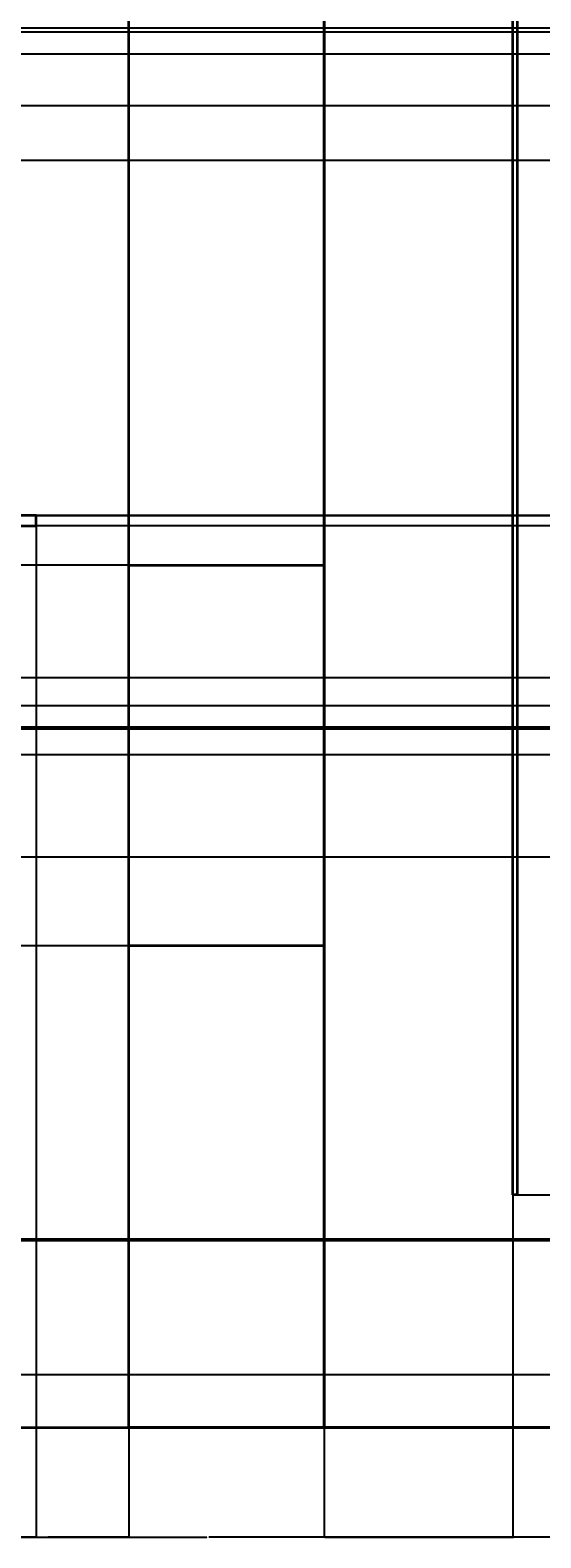
# Model space of a CAD drawing. Units: feet. Extents: x 4092 to 5585, y 725 to 1390.
# Tile 5 of 7: x 5204 to 5346, y 725 to 1146. Entities that reach past the tile are written whole.
import ezdxf

# ---------------------------------------------------------------- set-up
doc = ezdxf.new("R2010")
doc.units = ezdxf.units.FT
doc.layers.add('A-ANNO-DIMS', color=2, linetype='Continuous', lineweight=18)
doc.layers.add('A-ELEV', color=7, linetype='Continuous', lineweight=35)
doc.styles.get("Standard").update_dxf_attribs({"font": 'arial.ttf'})
doc.dimstyles.get("Standard").update_dxf_attribs({"dimtxt": 0.18, "dimasz": 0.18, "dimexe": 0.18, "dimexo": 0.0625, "dimgap": 0.09, "dimtad": 0, "dimtih": 1, "dimtoh": 1, "dimdec": 1, "dimzin": 0, "dimdsep": 46, "dimlunit": 3, "dimtxsty": 'Standard', "dimcen": 0.09, "dimadec": 0, "dimazin": 0, "dimtfac": 1, "dimtdec": 1, "dimtofl": 0, "dimtmove": 0, "dimatfit": 3, "dimfxl": 1, "dimtolj": 1, "dimtzin": 0, "dimarcsym": 0})

# ---------------------------------------------------------------- blocks, each defined once
blk = doc.blocks.new('*D4')
at = {"layer": 'A-ANNO-DIMS', "color": 0, "lineweight": -2, "transparency": 16777216}
for p, q in [((4953.29, 755.89), (4953.29, 725.07)), ((5553.29, 755.89), (5553.29, 725.07)), ((4953.47, 725.25), (5253, 725.25)), ((5553.11, 725.25), (5253.58, 725.25))]:
    blk.add_line(p, q, dxfattribs=at)
at = {"layer": 'A-ANNO-DIMS', "color": 0, "transparency": 16777216}
for points in [[(4953.47, 725.28), (4953.47, 725.22), (4953.29, 725.25)], [(5553.11, 725.28), (5553.11, 725.22), (5553.29, 725.25)]]:
    blk.add_solid(points, dxfattribs=at)
at = {"layer": 'Defpoints', "color": 0, "transparency": 16777216}
for p in [(4953.29, 755.95), (5553.29, 755.95), (5553.29, 725.25)]:
    blk.add_point(p, dxfattribs=at)
at = {"layer": 'A-ANNO-DIMS', "color": 0, "transparency": 16777216, "insert": (5253.29, 725.25), "char_height": 0.18, "attachment_point": 5}
blk.add_mtext('\\A1;600', dxfattribs=at)
blk = doc.blocks.new('*D5')
at = {"layer": 'A-ANNO-DIMS', "color": 0, "lineweight": -2, "transparency": 16777216}
for p, q in [((5264.26, 1358.97), (5584.71, 1358.97)), ((5584.53, 1358.79), (5584.53, 1057.64)), ((5584.53, 756.13), (5584.53, 1057.28)), ((5553.36, 755.95), (5584.71, 755.95))]:
    blk.add_line(p, q, dxfattribs=at)
at = {"layer": 'A-ANNO-DIMS', "color": 0, "transparency": 16777216}
for points in [[(5584.5, 1358.79), (5584.56, 1358.79), (5584.53, 1358.97)], [(5584.5, 756.13), (5584.56, 756.13), (5584.53, 755.95)]]:
    blk.add_solid(points, dxfattribs=at)
at = {"layer": 'Defpoints', "color": 0, "transparency": 16777216}
for p in [(5264.2, 1358.97), (5584.53, 1358.97), (5553.29, 755.95)]:
    blk.add_point(p, dxfattribs=at)
at = {"layer": 'A-ANNO-DIMS', "color": 0, "transparency": 16777216, "insert": (5584.53, 1057.46), "char_height": 0.18, "attachment_point": 5}
blk.add_mtext('\\A1;603', dxfattribs=at)
blk = doc.blocks.new('*D17')
at = {"layer": 'A-ANNO-DIMS', "color": 0, "lineweight": -2, "transparency": 16777216}
for p, q in [((5021.54, 951.2), (4921.27, 951.2)), ((4921.45, 951.02), (4921.45, 853.76)), ((4921.45, 756.13), (4921.45, 853.39)), ((5285.73, 755.95), (4921.27, 755.95))]:
    blk.add_line(p, q, dxfattribs=at)
at = {"layer": 'A-ANNO-DIMS', "color": 0, "transparency": 16777216}
for points in [[(4921.42, 951.02), (4921.48, 951.02), (4921.45, 951.2)], [(4921.42, 756.13), (4921.48, 756.13), (4921.45, 755.95)]]:
    blk.add_solid(points, dxfattribs=at)
at = {"layer": 'Defpoints', "color": 0, "transparency": 16777216}
for p in [(4921.45, 951.2), (5021.61, 951.2), (5285.79, 755.95)]:
    blk.add_point(p, dxfattribs=at)
at = {"layer": 'A-ANNO-DIMS', "color": 0, "transparency": 16777216, "insert": (4921.45, 853.58), "char_height": 0.18, "attachment_point": 5}
blk.add_mtext('\\A1;195.25', dxfattribs=at)
blk = doc.blocks.new('*D32')
at = {"layer": 'A-ANNO-DIMS', "color": 0, "lineweight": -2, "transparency": 16777216}
for p, q in [((5185.33, 755.89), (5185.33, 725.07)), ((5231.15, 755.89), (5231.15, 725.07)), ((5185.51, 725.25), (5207.84, 725.25)), ((5230.97, 725.25), (5208.64, 725.25))]:
    blk.add_line(p, q, dxfattribs=at)
at = {"layer": 'A-ANNO-DIMS', "color": 0, "transparency": 16777216}
for points in [[(5185.51, 725.28), (5185.51, 725.22), (5185.33, 725.25)], [(5230.97, 725.28), (5230.97, 725.22), (5231.15, 725.25)]]:
    blk.add_solid(points, dxfattribs=at)
at = {"layer": 'Defpoints', "color": 0, "transparency": 16777216}
for p in [(5185.33, 755.95), (5231.15, 755.95), (5231.15, 725.25)]:
    blk.add_point(p, dxfattribs=at)
at = {"layer": 'A-ANNO-DIMS', "color": 0, "transparency": 16777216, "insert": (5208.24, 725.25), "char_height": 0.18, "attachment_point": 5}
blk.add_mtext('\\A1;45.82', dxfattribs=at)
blk = doc.blocks.new('*D33')
at = {"layer": 'A-ANNO-DIMS', "color": 0, "lineweight": -2, "transparency": 16777216}
for p, q in [((5153.4, 808.21), (5584.71, 808.21)), ((5584.53, 808.03), (5584.53, 782.26)), ((5584.53, 756.13), (5584.53, 781.9)), ((5153.4, 755.95), (5584.71, 755.95))]:
    blk.add_line(p, q, dxfattribs=at)
at = {"layer": 'A-ANNO-DIMS', "color": 0, "transparency": 16777216}
for points in [[(5584.5, 808.03), (5584.56, 808.03), (5584.53, 808.21)], [(5584.5, 756.13), (5584.56, 756.13), (5584.53, 755.95)]]:
    blk.add_solid(points, dxfattribs=at)
at = {"layer": 'Defpoints', "color": 0, "transparency": 16777216}
for p in [(5153.34, 808.21), (5584.53, 808.21), (5153.34, 755.95)]:
    blk.add_point(p, dxfattribs=at)
at = {"layer": 'A-ANNO-DIMS', "color": 0, "transparency": 16777216, "insert": (5584.53, 782.08), "char_height": 0.18, "attachment_point": 5}
blk.add_mtext('\\A1;52.27', dxfattribs=at)
blk = doc.blocks.new('*D34')
at = {"layer": 'A-ANNO-DIMS', "color": 0, "lineweight": -2, "transparency": 16777216}
for p, q in [((5153.4, 915.42), (5584.71, 915.42)), ((5584.53, 915.24), (5584.53, 862)), ((5584.53, 808.39), (5584.53, 861.63)), ((5153.4, 808.21), (5584.71, 808.21))]:
    blk.add_line(p, q, dxfattribs=at)
at = {"layer": 'A-ANNO-DIMS', "color": 0, "transparency": 16777216}
for points in [[(5584.5, 915.24), (5584.56, 915.24), (5584.53, 915.42)], [(5584.5, 808.39), (5584.56, 808.39), (5584.53, 808.21)]]:
    blk.add_solid(points, dxfattribs=at)
at = {"layer": 'Defpoints', "color": 0, "transparency": 16777216}
for p in [(5153.34, 915.42), (5584.53, 915.42), (5153.34, 808.21)]:
    blk.add_point(p, dxfattribs=at)
at = {"layer": 'A-ANNO-DIMS', "color": 0, "transparency": 16777216, "insert": (5584.53, 861.82), "char_height": 0.18, "attachment_point": 5}
blk.add_mtext('\\A1;107.2', dxfattribs=at)
blk = doc.blocks.new('*D35')
at = {"layer": 'A-ANNO-DIMS', "color": 0, "lineweight": -2, "transparency": 16777216}
for p, q in [((5153.4, 944.01), (5584.71, 944.01)), ((5584.53, 943.83), (5584.53, 929.9)), ((5584.53, 915.6), (5584.53, 929.53)), ((5153.4, 915.42), (5584.71, 915.42))]:
    blk.add_line(p, q, dxfattribs=at)
at = {"layer": 'A-ANNO-DIMS', "color": 0, "transparency": 16777216}
for points in [[(5584.5, 943.83), (5584.56, 943.83), (5584.53, 944.01)], [(5584.5, 915.6), (5584.56, 915.6), (5584.53, 915.42)]]:
    blk.add_solid(points, dxfattribs=at)
at = {"layer": 'Defpoints', "color": 0, "transparency": 16777216}
for p in [(5153.34, 944.01), (5584.53, 944.01), (5153.34, 915.42)]:
    blk.add_point(p, dxfattribs=at)
at = {"layer": 'A-ANNO-DIMS', "color": 0, "transparency": 16777216, "insert": (5584.53, 929.71), "char_height": 0.18, "attachment_point": 5}
blk.add_mtext('\\A1;28.59', dxfattribs=at)
blk = doc.blocks.new('*D36')
at = {"layer": 'A-ANNO-DIMS', "color": 0, "lineweight": -2, "transparency": 16777216}
for p, q in [((5160.6, 951.2), (5584.71, 951.2)), ((5584.53, 951.02), (5584.53, 947.79)), ((5153.4, 944.01), (5584.71, 944.01)), ((5584.53, 944.19), (5584.53, 947.42))]:
    blk.add_line(p, q, dxfattribs=at)
at = {"layer": 'A-ANNO-DIMS', "color": 0, "transparency": 16777216}
for points in [[(5584.5, 951.02), (5584.56, 951.02), (5584.53, 951.2)], [(5584.5, 944.19), (5584.56, 944.19), (5584.53, 944.01)]]:
    blk.add_solid(points, dxfattribs=at)
at = {"layer": 'Defpoints', "color": 0, "transparency": 16777216}
for p in [(5160.53, 951.2), (5584.53, 951.2), (5153.34, 944.01)]:
    blk.add_point(p, dxfattribs=at)
at = {"layer": 'A-ANNO-DIMS', "color": 0, "transparency": 16777216, "insert": (5584.53, 947.61), "char_height": 0.18, "attachment_point": 5}
blk.add_mtext('\\A1;7.194', dxfattribs=at)
blk = doc.blocks.new('*D37')
at = {"layer": 'A-ANNO-DIMS', "color": 0, "lineweight": -2, "transparency": 16777216}
for p, q in [((5094.36, 770.68), (5584.71, 770.68)), ((5584.53, 770.5), (5584.53, 763.5)), ((5584.53, 756.13), (5584.53, 763.13)), ((5057.45, 755.95), (5584.71, 755.95))]:
    blk.add_line(p, q, dxfattribs=at)
at = {"layer": 'A-ANNO-DIMS', "color": 0, "transparency": 16777216}
for points in [[(5584.5, 770.5), (5584.56, 770.5), (5584.53, 770.68)], [(5584.5, 756.13), (5584.56, 756.13), (5584.53, 755.95)]]:
    blk.add_solid(points, dxfattribs=at)
at = {"layer": 'Defpoints', "color": 0, "transparency": 16777216}
for p in [(5094.3, 770.68), (5584.53, 770.68), (5057.39, 755.95)]:
    blk.add_point(p, dxfattribs=at)
at = {"layer": 'A-ANNO-DIMS', "color": 0, "transparency": 16777216, "insert": (5584.53, 763.31), "char_height": 0.18, "attachment_point": 5}
blk.add_mtext('\\A1;14.73', dxfattribs=at)
blk = doc.blocks.new('*D38')
at = {"layer": 'A-ANNO-DIMS', "color": 0, "lineweight": -2, "transparency": 16777216}
for p, q in [((5094.36, 808.65), (5584.71, 808.65)), ((5584.53, 808.47), (5584.53, 789.85)), ((5584.53, 770.86), (5584.53, 789.48)), ((5094.36, 770.68), (5584.71, 770.68))]:
    blk.add_line(p, q, dxfattribs=at)
at = {"layer": 'A-ANNO-DIMS', "color": 0, "transparency": 16777216}
for points in [[(5584.5, 808.47), (5584.56, 808.47), (5584.53, 808.65)], [(5584.5, 770.86), (5584.56, 770.86), (5584.53, 770.68)]]:
    blk.add_solid(points, dxfattribs=at)
at = {"layer": 'Defpoints', "color": 0, "transparency": 16777216}
for p in [(5094.3, 808.65), (5584.53, 808.65), (5094.3, 770.68)]:
    blk.add_point(p, dxfattribs=at)
at = {"layer": 'A-ANNO-DIMS', "color": 0, "transparency": 16777216, "insert": (5584.53, 789.67), "char_height": 0.18, "attachment_point": 5}
blk.add_mtext('\\A1;37.97', dxfattribs=at)
blk = doc.blocks.new('*D56')
at = {"layer": 'A-ANNO-DIMS', "color": 0, "lineweight": -2, "transparency": 16777216}
for p, q in [((5185.33, 1010.73), (5185.33, 725.07)), ((5205.28, 1010.73), (5205.28, 725.07)), ((5185.51, 725.25), (5194.85, 725.25)), ((5205.1, 725.25), (5195.76, 725.25))]:
    blk.add_line(p, q, dxfattribs=at)
at = {"layer": 'A-ANNO-DIMS', "color": 0, "transparency": 16777216}
for points in [[(5185.51, 725.28), (5185.51, 725.22), (5185.33, 725.25)], [(5205.1, 725.28), (5205.1, 725.22), (5205.28, 725.25)]]:
    blk.add_solid(points, dxfattribs=at)
at = {"layer": 'Defpoints', "color": 0, "transparency": 16777216}
for p in [(5185.33, 1010.79), (5205.28, 1010.79), (5205.28, 725.25)]:
    blk.add_point(p, dxfattribs=at)
at = {"layer": 'A-ANNO-DIMS', "color": 0, "transparency": 16777216, "insert": (5195.3, 725.25), "char_height": 0.18, "attachment_point": 5}
blk.add_mtext('\\A1;19.947', dxfattribs=at)
blk = doc.blocks.new('*D57')
at = {"layer": 'A-ANNO-DIMS', "color": 0, "lineweight": -2, "transparency": 16777216}
for p, q in [((5153.4, 1110.12), (5584.71, 1110.12)), ((5584.53, 1109.94), (5584.53, 1060.64)), ((5584.53, 1010.97), (5584.53, 1060.27)), ((5185.39, 1010.79), (5584.71, 1010.79))]:
    blk.add_line(p, q, dxfattribs=at)
at = {"layer": 'A-ANNO-DIMS', "color": 0, "transparency": 16777216}
for points in [[(5584.5, 1109.94), (5584.56, 1109.94), (5584.53, 1110.12)], [(5584.5, 1010.97), (5584.56, 1010.97), (5584.53, 1010.79)]]:
    blk.add_solid(points, dxfattribs=at)
at = {"layer": 'Defpoints', "color": 0, "transparency": 16777216}
for p in [(5153.34, 1110.12), (5584.53, 1110.12), (5185.33, 1010.79)]:
    blk.add_point(p, dxfattribs=at)
at = {"layer": 'A-ANNO-DIMS', "color": 0, "transparency": 16777216, "insert": (5584.53, 1060.45), "char_height": 0.18, "attachment_point": 5}
blk.add_mtext('\\A1;99.33', dxfattribs=at)
blk = doc.blocks.new('*D58')
at = {"layer": 'A-ANNO-DIMS', "color": 0, "lineweight": -2, "transparency": 16777216}
for p, q in [((5153.4, 1139.88), (5584.71, 1139.88)), ((5584.53, 1139.7), (5584.53, 1125.18)), ((5584.53, 1110.3), (5584.53, 1124.82)), ((5153.4, 1110.12), (5584.71, 1110.12))]:
    blk.add_line(p, q, dxfattribs=at)
at = {"layer": 'A-ANNO-DIMS', "color": 0, "transparency": 16777216}
for points in [[(5584.5, 1139.7), (5584.56, 1139.7), (5584.53, 1139.88)], [(5584.5, 1110.3), (5584.56, 1110.3), (5584.53, 1110.12)]]:
    blk.add_solid(points, dxfattribs=at)
at = {"layer": 'Defpoints', "color": 0, "transparency": 16777216}
for p in [(5153.34, 1139.88), (5584.53, 1139.88), (5153.34, 1110.12)]:
    blk.add_point(p, dxfattribs=at)
at = {"layer": 'A-ANNO-DIMS', "color": 0, "transparency": 16777216, "insert": (5584.53, 1125), "char_height": 0.18, "attachment_point": 5}
blk.add_mtext('\\A1;29.76', dxfattribs=at)
blk = doc.blocks.new('*D59')
at = {"layer": 'A-ANNO-DIMS', "color": 0, "lineweight": -2, "transparency": 16777216}
for p, q in [((5185.39, 1147.07), (5584.71, 1147.07)), ((5584.53, 1146.89), (5584.53, 1143.66)), ((5584.53, 1140.06), (5584.53, 1143.3)), ((5153.4, 1139.88), (5584.71, 1139.88))]:
    blk.add_line(p, q, dxfattribs=at)
at = {"layer": 'A-ANNO-DIMS', "color": 0, "transparency": 16777216}
for points in [[(5584.5, 1146.89), (5584.56, 1146.89), (5584.53, 1147.07)], [(5584.5, 1140.06), (5584.56, 1140.06), (5584.53, 1139.88)]]:
    blk.add_solid(points, dxfattribs=at)
at = {"layer": 'Defpoints', "color": 0, "transparency": 16777216}
for p in [(5185.33, 1147.07), (5584.53, 1147.07), (5153.34, 1139.88)]:
    blk.add_point(p, dxfattribs=at)
at = {"layer": 'A-ANNO-DIMS', "color": 0, "transparency": 16777216, "insert": (5584.53, 1143.48), "char_height": 0.18, "attachment_point": 5}
blk.add_mtext('\\A1;7.194', dxfattribs=at)
blk = doc.blocks.new('*D64')
at = {"layer": 'A-ANNO-DIMS', "color": 0, "lineweight": -2, "transparency": 16777216}
for p, q in [((5285.79, 755.89), (5285.79, 725.07)), ((5392.55, 755.89), (5392.55, 725.07)), ((5285.97, 725.25), (5338.72, 725.25)), ((5392.37, 725.25), (5339.63, 725.25))]:
    blk.add_line(p, q, dxfattribs=at)
at = {"layer": 'A-ANNO-DIMS', "color": 0, "transparency": 16777216}
for points in [[(5285.97, 725.28), (5285.97, 725.22), (5285.79, 725.25)], [(5392.37, 725.28), (5392.37, 725.22), (5392.55, 725.25)]]:
    blk.add_solid(points, dxfattribs=at)
at = {"layer": 'Defpoints', "color": 0, "transparency": 16777216}
for p in [(5285.79, 755.95), (5392.55, 755.95), (5392.55, 725.25)]:
    blk.add_point(p, dxfattribs=at)
at = {"layer": 'A-ANNO-DIMS', "color": 0, "transparency": 16777216, "insert": (5339.17, 725.25), "char_height": 0.18, "attachment_point": 5}
blk.add_mtext('\\A1;106.76', dxfattribs=at)
blk = doc.blocks.new('*D71')
at = {"layer": 'A-ANNO-DIMS', "color": 0, "lineweight": -2, "transparency": 16777216}
for p, q in [((5285.73, 890.54), (4921.27, 890.54)), ((4921.45, 890.36), (4921.45, 823.43)), ((4921.45, 756.13), (4921.45, 823.06)), ((5285.73, 755.95), (4921.27, 755.95))]:
    blk.add_line(p, q, dxfattribs=at)
at = {"layer": 'A-ANNO-DIMS', "color": 0, "transparency": 16777216}
for points in [[(4921.42, 890.36), (4921.48, 890.36), (4921.45, 890.54)], [(4921.42, 756.13), (4921.48, 756.13), (4921.45, 755.95)]]:
    blk.add_solid(points, dxfattribs=at)
at = {"layer": 'Defpoints', "color": 0, "transparency": 16777216}
for p in [(4921.45, 890.54), (5285.79, 890.54), (5285.79, 755.95)]:
    blk.add_point(p, dxfattribs=at)
at = {"layer": 'A-ANNO-DIMS', "color": 0, "transparency": 16777216, "insert": (4921.45, 823.24), "char_height": 0.18, "attachment_point": 5}
blk.add_mtext('\\A1;134.6', dxfattribs=at)
blk = doc.blocks.new('*D72')
at = {"layer": 'A-ANNO-DIMS', "color": 0, "lineweight": -2, "transparency": 16777216}
for p, q in [((5285.73, 996.97), (4921.27, 996.97)), ((4921.45, 996.79), (4921.45, 943.94)), ((4921.45, 890.72), (4921.45, 943.57)), ((5285.73, 890.54), (4921.27, 890.54))]:
    blk.add_line(p, q, dxfattribs=at)
at = {"layer": 'A-ANNO-DIMS', "color": 0, "transparency": 16777216}
for points in [[(4921.42, 996.79), (4921.48, 996.79), (4921.45, 996.97)], [(4921.42, 890.72), (4921.48, 890.72), (4921.45, 890.54)]]:
    blk.add_solid(points, dxfattribs=at)
at = {"layer": 'Defpoints', "color": 0, "transparency": 16777216}
for p in [(4921.45, 996.97), (5285.79, 996.97), (5285.79, 890.54)]:
    blk.add_point(p, dxfattribs=at)
at = {"layer": 'A-ANNO-DIMS', "color": 0, "transparency": 16777216, "insert": (4921.45, 943.75), "char_height": 0.18, "attachment_point": 5}
blk.add_mtext('\\A1;106.43', dxfattribs=at)
blk = doc.blocks.new('*D73')
at = {"layer": 'A-ANNO-DIMS', "color": 0, "lineweight": -2, "transparency": 16777216}
for p, q in [((5339.81, 820.92), (5584.71, 820.92)), ((5584.53, 820.74), (5584.53, 788.62)), ((5584.53, 756.13), (5584.53, 788.25)), ((5285.85, 755.95), (5584.71, 755.95))]:
    blk.add_line(p, q, dxfattribs=at)
at = {"layer": 'A-ANNO-DIMS', "color": 0, "transparency": 16777216}
for points in [[(5584.5, 820.74), (5584.56, 820.74), (5584.53, 820.92)], [(5584.5, 756.13), (5584.56, 756.13), (5584.53, 755.95)]]:
    blk.add_solid(points, dxfattribs=at)
at = {"layer": 'Defpoints', "color": 0, "transparency": 16777216}
for p in [(5339.75, 820.92), (5584.53, 820.92), (5285.79, 755.95)]:
    blk.add_point(p, dxfattribs=at)
at = {"layer": 'A-ANNO-DIMS', "color": 0, "transparency": 16777216, "insert": (5584.53, 788.43), "char_height": 0.18, "attachment_point": 5}
blk.add_mtext('\\A1;64.97', dxfattribs=at)
blk = doc.blocks.new('*D74')
at = {"layer": 'A-ANNO-DIMS', "color": 0, "lineweight": -2, "transparency": 16777216}
for p, q in [((5285.79, 890.48), (5285.79, 725.07)), ((5338.59, 820.86), (5338.59, 725.07)), ((5285.97, 725.25), (5311.87, 725.25)), ((5338.41, 725.25), (5312.52, 725.25))]:
    blk.add_line(p, q, dxfattribs=at)
at = {"layer": 'A-ANNO-DIMS', "color": 0, "transparency": 16777216}
for points in [[(5285.97, 725.28), (5285.97, 725.22), (5285.79, 725.25)], [(5338.41, 725.28), (5338.41, 725.22), (5338.59, 725.25)]]:
    blk.add_solid(points, dxfattribs=at)
at = {"layer": 'Defpoints', "color": 0, "transparency": 16777216}
for p in [(5285.79, 890.54), (5338.59, 820.92), (5338.59, 725.25)]:
    blk.add_point(p, dxfattribs=at)
at = {"layer": 'A-ANNO-DIMS', "color": 0, "transparency": 16777216, "insert": (5312.19, 725.25), "char_height": 0.18, "attachment_point": 5}
blk.add_mtext('\\A1;52.8', dxfattribs=at)
blk = doc.blocks.new('*D75')
at = {"layer": 'A-ANNO-DIMS', "color": 0, "lineweight": -2, "transparency": 16777216}
for p, q in [((5392.49, 951.65), (4921.27, 951.65)), ((4921.45, 951.47), (4921.45, 853.98)), ((4921.45, 756.13), (4921.45, 853.62)), ((5392.49, 755.95), (4921.27, 755.95))]:
    blk.add_line(p, q, dxfattribs=at)
at = {"layer": 'A-ANNO-DIMS', "color": 0, "transparency": 16777216}
for points in [[(4921.42, 951.47), (4921.48, 951.47), (4921.45, 951.65)], [(4921.42, 756.13), (4921.48, 756.13), (4921.45, 755.95)]]:
    blk.add_solid(points, dxfattribs=at)
at = {"layer": 'Defpoints', "color": 0, "transparency": 16777216}
for p in [(4921.45, 951.65), (5392.55, 951.65), (5392.55, 755.95)]:
    blk.add_point(p, dxfattribs=at)
at = {"layer": 'A-ANNO-DIMS', "color": 0, "transparency": 16777216, "insert": (4921.45, 853.8), "char_height": 0.18, "attachment_point": 5}
blk.add_mtext('\\A1;195.7', dxfattribs=at)
blk = doc.blocks.new('*D76')
at = {"layer": 'A-ANNO-DIMS', "color": 0, "lineweight": -2, "transparency": 16777216}
for p, q in [((5392.49, 957.65), (4921.27, 957.65)), ((4921.45, 957.47), (4921.45, 954.83)), ((4921.45, 951.83), (4921.45, 954.46)), ((5392.49, 951.65), (4921.27, 951.65))]:
    blk.add_line(p, q, dxfattribs=at)
at = {"layer": 'A-ANNO-DIMS', "color": 0, "transparency": 16777216}
for points in [[(4921.42, 957.47), (4921.48, 957.47), (4921.45, 957.65)], [(4921.42, 951.83), (4921.48, 951.83), (4921.45, 951.65)]]:
    blk.add_solid(points, dxfattribs=at)
at = {"layer": 'Defpoints', "color": 0, "transparency": 16777216}
for p in [(4921.45, 957.65), (5392.55, 957.65), (5392.55, 951.65)]:
    blk.add_point(p, dxfattribs=at)
at = {"layer": 'A-ANNO-DIMS', "color": 0, "transparency": 16777216, "insert": (4921.45, 954.65), "char_height": 0.18, "attachment_point": 5}
blk.add_mtext('\\A1;6', dxfattribs=at)
blk = doc.blocks.new('*D77')
at = {"layer": 'A-ANNO-DIMS', "color": 0, "lineweight": -2, "transparency": 16777216}
for p, q in [((5392.49, 965.48), (4921.27, 965.48)), ((4921.45, 965.3), (4921.45, 961.74)), ((4921.45, 957.83), (4921.45, 961.38)), ((5392.49, 957.65), (4921.27, 957.65))]:
    blk.add_line(p, q, dxfattribs=at)
at = {"layer": 'A-ANNO-DIMS', "color": 0, "transparency": 16777216}
for points in [[(4921.42, 965.3), (4921.48, 965.3), (4921.45, 965.48)], [(4921.42, 957.83), (4921.48, 957.83), (4921.45, 957.65)]]:
    blk.add_solid(points, dxfattribs=at)
at = {"layer": 'Defpoints', "color": 0, "transparency": 16777216}
for p in [(4921.45, 965.48), (5392.55, 965.48), (5392.55, 957.65)]:
    blk.add_point(p, dxfattribs=at)
at = {"layer": 'A-ANNO-DIMS', "color": 0, "transparency": 16777216, "insert": (4921.45, 961.56), "char_height": 0.18, "attachment_point": 5}
blk.add_mtext('\\A1;7.833', dxfattribs=at)
blk = doc.blocks.new('*D78')
at = {"layer": 'A-ANNO-DIMS', "color": 0, "lineweight": -2, "transparency": 16777216}
for p, q in [((5392.49, 1007.95), (4921.27, 1007.95)), ((4921.45, 1007.77), (4921.45, 986.89)), ((4921.45, 965.66), (4921.45, 986.53)), ((5392.49, 965.48), (4921.27, 965.48))]:
    blk.add_line(p, q, dxfattribs=at)
at = {"layer": 'A-ANNO-DIMS', "color": 0, "transparency": 16777216}
for points in [[(4921.42, 1007.77), (4921.48, 1007.77), (4921.45, 1007.95)], [(4921.42, 965.66), (4921.48, 965.66), (4921.45, 965.48)]]:
    blk.add_solid(points, dxfattribs=at)
at = {"layer": 'Defpoints', "color": 0, "transparency": 16777216}
for p in [(4921.45, 1007.95), (5392.55, 1007.95), (5392.55, 965.48)]:
    blk.add_point(p, dxfattribs=at)
at = {"layer": 'A-ANNO-DIMS', "color": 0, "transparency": 16777216, "insert": (4921.45, 986.71), "char_height": 0.18, "attachment_point": 5}
blk.add_mtext('\\A1;42.47', dxfattribs=at)
blk = doc.blocks.new('*D79')
at = {"layer": 'A-ANNO-DIMS', "color": 0, "lineweight": -2, "transparency": 16777216}
for p, q in [((5392.49, 1125.34), (4921.27, 1125.34)), ((4921.45, 1125.16), (4921.45, 1068.25)), ((4921.45, 1010.97), (4921.45, 1067.88)), ((5392.49, 1010.79), (4921.27, 1010.79))]:
    blk.add_line(p, q, dxfattribs=at)
at = {"layer": 'A-ANNO-DIMS', "color": 0, "transparency": 16777216}
for points in [[(4921.42, 1125.16), (4921.48, 1125.16), (4921.45, 1125.34)], [(4921.42, 1010.97), (4921.48, 1010.97), (4921.45, 1010.79)]]:
    blk.add_solid(points, dxfattribs=at)
at = {"layer": 'Defpoints', "color": 0, "transparency": 16777216}
for p in [(4921.45, 1125.34), (5392.55, 1125.34), (5392.55, 1010.79)]:
    blk.add_point(p, dxfattribs=at)
at = {"layer": 'A-ANNO-DIMS', "color": 0, "transparency": 16777216, "insert": (4921.45, 1068.07), "char_height": 0.18, "attachment_point": 5}
blk.add_mtext('\\A1;114.55', dxfattribs=at)
blk = doc.blocks.new('*D80')
at = {"layer": 'A-ANNO-DIMS', "color": 0, "lineweight": -2, "transparency": 16777216}
for p, q in [((5392.49, 1145.86), (4921.27, 1145.86)), ((4921.45, 1145.68), (4921.45, 1135.78)), ((4921.45, 1125.52), (4921.45, 1135.42)), ((5392.49, 1125.34), (4921.27, 1125.34))]:
    blk.add_line(p, q, dxfattribs=at)
at = {"layer": 'A-ANNO-DIMS', "color": 0, "transparency": 16777216}
for points in [[(4921.42, 1145.68), (4921.48, 1145.68), (4921.45, 1145.86)], [(4921.42, 1125.52), (4921.48, 1125.52), (4921.45, 1125.34)]]:
    blk.add_solid(points, dxfattribs=at)
at = {"layer": 'Defpoints', "color": 0, "transparency": 16777216}
for p in [(4921.45, 1145.86), (5392.55, 1145.86), (5392.55, 1125.34)]:
    blk.add_point(p, dxfattribs=at)
at = {"layer": 'A-ANNO-DIMS', "color": 0, "transparency": 16777216, "insert": (4921.45, 1135.6), "char_height": 0.18, "attachment_point": 5}
blk.add_mtext('\\A1;20.52', dxfattribs=at)
blk = doc.blocks.new('*D81')
at = {"layer": 'A-ANNO-DIMS', "color": 0, "lineweight": -2, "transparency": 16777216}
for p, q in [((5392.49, 1171.51), (4921.27, 1171.51)), ((4921.45, 1171.33), (4921.45, 1158.87)), ((4921.45, 1146.04), (4921.45, 1158.5)), ((5392.49, 1145.86), (4921.27, 1145.86))]:
    blk.add_line(p, q, dxfattribs=at)
at = {"layer": 'A-ANNO-DIMS', "color": 0, "transparency": 16777216}
for points in [[(4921.42, 1171.33), (4921.48, 1171.33), (4921.45, 1171.51)], [(4921.42, 1146.04), (4921.48, 1146.04), (4921.45, 1145.86)]]:
    blk.add_solid(points, dxfattribs=at)
at = {"layer": 'Defpoints', "color": 0, "transparency": 16777216}
for p in [(4921.45, 1171.51), (5392.55, 1171.51), (5392.55, 1145.86)]:
    blk.add_point(p, dxfattribs=at)
at = {"layer": 'A-ANNO-DIMS', "color": 0, "transparency": 16777216, "insert": (4921.45, 1158.69), "char_height": 0.18, "attachment_point": 5}
blk.add_mtext('\\A1;25.65', dxfattribs=at)

msp = doc.modelspace()

# ---------------------------------------------------------------- linework, layer by layer
at = {"layer": 'A-ELEV'}
msp.add_line((4953.293, 755.9488), (5553.293, 755.9488), dxfattribs=at)
for points in [[(5392.5521, 755.9488), (5285.7915, 755.9488), (5285.7915, 1305.7746), (5392.5521, 1305.7746)], [(5338.5913, 820.9207), (5338.5913, 1258.8497), (5339.7523, 1258.8497), (5339.7523, 820.9207)], [(4953.293, 755.9488), (5231.15, 755.9488), (5231.15, 1253.9488), (4953.293, 1253.9488)], [(5231.15, 1253.9488), (5285.7915, 1253.9488), (5285.7915, 755.9488), (5231.15, 755.9488)], [(4978.356, 1007.9488), (5205.2757, 1007.9488), (5205.2757, 1010.7906), (4978.356, 1010.7906)], [(5231.15, 996.9712), (5285.7915, 996.9712), (5285.7915, 890.5384), (5231.15, 890.5384)]]:
    msp.add_lwpolyline(points, close=True, dxfattribs=at)

# ---------------------------------------------------------------- dimensions: what is measured, and where the dimension line sits
at = {"layer": 'A-ANNO-DIMS'}
for base, p1, p2, override, picture, middle in [((5584.5322, 1358.9731), (5553.293, 755.9488), (5264.1979, 1358.9731), {"dimdec": 0, "dimlfac": 1, "dimrnd": 0, "dimzin": 0, "dimdsep": 46, "dimlunit": 2}, '*D5', (5584.5322, 1057.461)), ((4921.4517, 1171.511), (5392.5521, 1145.8611), (5392.5521, 1171.511), {"dimdec": 2, "dimlfac": 1, "dimrnd": 0, "dimzin": 0, "dimdsep": 46, "dimlunit": 2}, '*D81', (4921.4517, 1158.6861)), ((5584.5322, 1147.0743), (5153.3388, 1139.8803), (5185.3285, 1147.0743), {"dimdec": 3, "dimlfac": 1, "dimrnd": 0, "dimzin": 0, "dimdsep": 46, "dimlunit": 2}, '*D59', (5584.5322, 1143.4773)), ((4921.4517, 1145.8611), (5392.5521, 1125.3426), (5392.5521, 1145.8611), {"dimdec": 2, "dimlfac": 1, "dimrnd": 0, "dimzin": 0, "dimdsep": 46, "dimlunit": 2}, '*D80', (4921.4517, 1135.6018)), ((5584.5322, 1139.8803), (5153.3388, 1110.119), (5153.3388, 1139.8803), {"dimdec": 2, "dimlfac": 1, "dimrnd": 0, "dimzin": 0, "dimdsep": 46, "dimlunit": 2}, '*D58', (5584.5322, 1124.9996)), ((4921.4517, 1125.3426), (5392.5521, 1010.7906), (5392.5521, 1125.3426), {"dimdec": 2, "dimlfac": 1, "dimrnd": 0, "dimzin": 0, "dimdsep": 46, "dimlunit": 2}, '*D79', (4921.4517, 1068.0666)), ((5584.5322, 1110.119), (5185.3285, 1010.7906), (5153.3388, 1110.119), {"dimdec": 2, "dimlfac": 1, "dimrnd": 0, "dimzin": 0, "dimdsep": 46, "dimlunit": 2}, '*D57', (5584.5322, 1060.4548)), ((4921.4517, 1007.9488), (5392.5521, 965.4789), (5392.5521, 1007.9488), {"dimdec": 2, "dimlfac": 1, "dimrnd": 0, "dimzin": 0, "dimdsep": 46, "dimlunit": 2}, '*D78', (4921.4517, 986.7139)), ((4921.4517, 996.9712), (5285.7915, 890.5384), (5285.7915, 996.9712), {"dimdec": 2, "dimlfac": 1, "dimrnd": 0, "dimzin": 0, "dimdsep": 46, "dimlunit": 2}, '*D72', (4921.4517, 943.7548)), ((4921.4517, 965.4789), (5392.5521, 957.6463), (5392.5521, 965.4789), {"dimdec": 3, "dimlfac": 1, "dimrnd": 0, "dimzin": 0, "dimdsep": 46, "dimlunit": 2}, '*D77', (4921.4517, 961.5626)), ((4921.4517, 957.6463), (5392.5521, 951.6463), (5392.5521, 957.6463), {"dimdec": 0, "dimlfac": 1, "dimrnd": 0, "dimzin": 0, "dimdsep": 46, "dimlunit": 2}, '*D76', (4921.4517, 954.6463)), ((4921.4517, 951.2024), (5285.7915, 755.9488), (5021.6062, 951.2024), {"dimdec": 2, "dimlfac": 1, "dimrnd": 0, "dimzin": 0, "dimdsep": 46, "dimlunit": 2}, '*D17', (4921.4517, 853.5756)), ((4921.4517, 951.6463), (5392.5521, 755.9488), (5392.5521, 951.6463), {"dimdec": 1, "dimlfac": 1, "dimrnd": 0, "dimzin": 0, "dimdsep": 46, "dimlunit": 2}, '*D75', (4921.4517, 853.7975)), ((5584.5322, 951.2024), (5153.3388, 944.0084), (5160.5329, 951.2024), {"dimdec": 3, "dimlfac": 1, "dimrnd": 0, "dimzin": 0, "dimdsep": 46, "dimlunit": 2}, '*D36', (5584.5322, 947.6054)), ((5584.5322, 944.0084), (5153.3388, 915.418), (5153.3388, 944.0084), {"dimdec": 2, "dimlfac": 1, "dimrnd": 0, "dimzin": 0, "dimdsep": 46, "dimlunit": 2}, '*D35', (5584.5322, 929.7132)), ((5584.5322, 915.418), (5153.3388, 808.2143), (5153.3388, 915.418), {"dimdec": 1, "dimlfac": 1, "dimrnd": 0, "dimzin": 0, "dimdsep": 46, "dimlunit": 2}, '*D34', (5584.5322, 861.8161)), ((4921.4517, 890.5384), (5285.7915, 755.9488), (5285.7915, 890.5384), {"dimdec": 1, "dimlfac": 1, "dimrnd": 0, "dimzin": 0, "dimdsep": 46, "dimlunit": 2}, '*D71', (4921.4517, 823.2436)), ((5584.5322, 820.9207), (5285.7915, 755.9488), (5339.7523, 820.9207), {"dimdec": 2, "dimlfac": 1, "dimrnd": 0, "dimzin": 0, "dimdsep": 46, "dimlunit": 2}, '*D73', (5584.5322, 788.4347)), ((5584.5322, 808.6527), (5094.3002, 770.6797), (5094.3002, 808.6527), {"dimdec": 2, "dimlfac": 1, "dimrnd": 0, "dimzin": 0, "dimdsep": 46, "dimlunit": 2}, '*D38', (5584.5322, 789.6662)), ((5584.5322, 808.2143), (5153.3388, 755.9488), (5153.3388, 808.2143), {"dimdec": 2, "dimlfac": 1, "dimrnd": 0, "dimzin": 0, "dimdsep": 46, "dimlunit": 2}, '*D33', (5584.5322, 782.0815)), ((5584.5322, 770.6797), (5057.3906, 755.9488), (5094.3002, 770.6797), {"dimdec": 2, "dimlfac": 1, "dimrnd": 0, "dimzin": 0, "dimdsep": 46, "dimlunit": 2}, '*D37', (5584.5322, 763.3143))]:
    dim = msp.add_linear_dim(base=base, p1=p1, p2=p2, angle=90, dimstyle='Standard', override=override, dxfattribs=at)
    dim.commit()
    dim.dimension.update_dxf_attribs({"geometry": picture, "text_midpoint": middle})
for base, p1, p2, override, picture, middle in [((5205.2757, 725.2488), (5185.3285, 1010.7906), (5205.2757, 1010.7906), {"dimdec": 3, "dimlfac": 1, "dimrnd": 0, "dimzin": 0, "dimdsep": 46, "dimlunit": 2}, '*D56', (5195.3021, 725.2488)), ((5338.5913, 725.2488), (5285.7915, 890.5384), (5338.5913, 820.9207), {"dimdec": 1, "dimlfac": 1, "dimrnd": 0, "dimzin": 0, "dimdsep": 46, "dimlunit": 2}, '*D74', (5312.1914, 725.2488)), ((5553.293, 725.2488), (4953.293, 755.9488), (5553.293, 755.9488), {"dimdec": 0, "dimlfac": 1, "dimrnd": 0, "dimzin": 0, "dimdsep": 46, "dimlunit": 2}, '*D4', (5253.293, 725.2488)), ((5231.15, 725.2488), (5185.3285, 755.9488), (5231.15, 755.9488), {"dimdec": 2, "dimlfac": 1, "dimrnd": 0, "dimzin": 0, "dimdsep": 46, "dimlunit": 2}, '*D32', (5208.2393, 725.2488)), ((5392.5521, 725.2488), (5285.7915, 755.9488), (5392.5521, 755.9488), {"dimdec": 2, "dimlfac": 1, "dimrnd": 0, "dimzin": 0, "dimdsep": 46, "dimlunit": 2}, '*D64', (5339.1718, 725.2488))]:
    dim = msp.add_linear_dim(base=base, p1=p1, p2=p2, dimstyle='Standard', override=override, dxfattribs=at)
    dim.commit()
    dim.dimension.update_dxf_attribs({"geometry": picture, "text_midpoint": middle})

doc.saveas('drawing.dxf')
